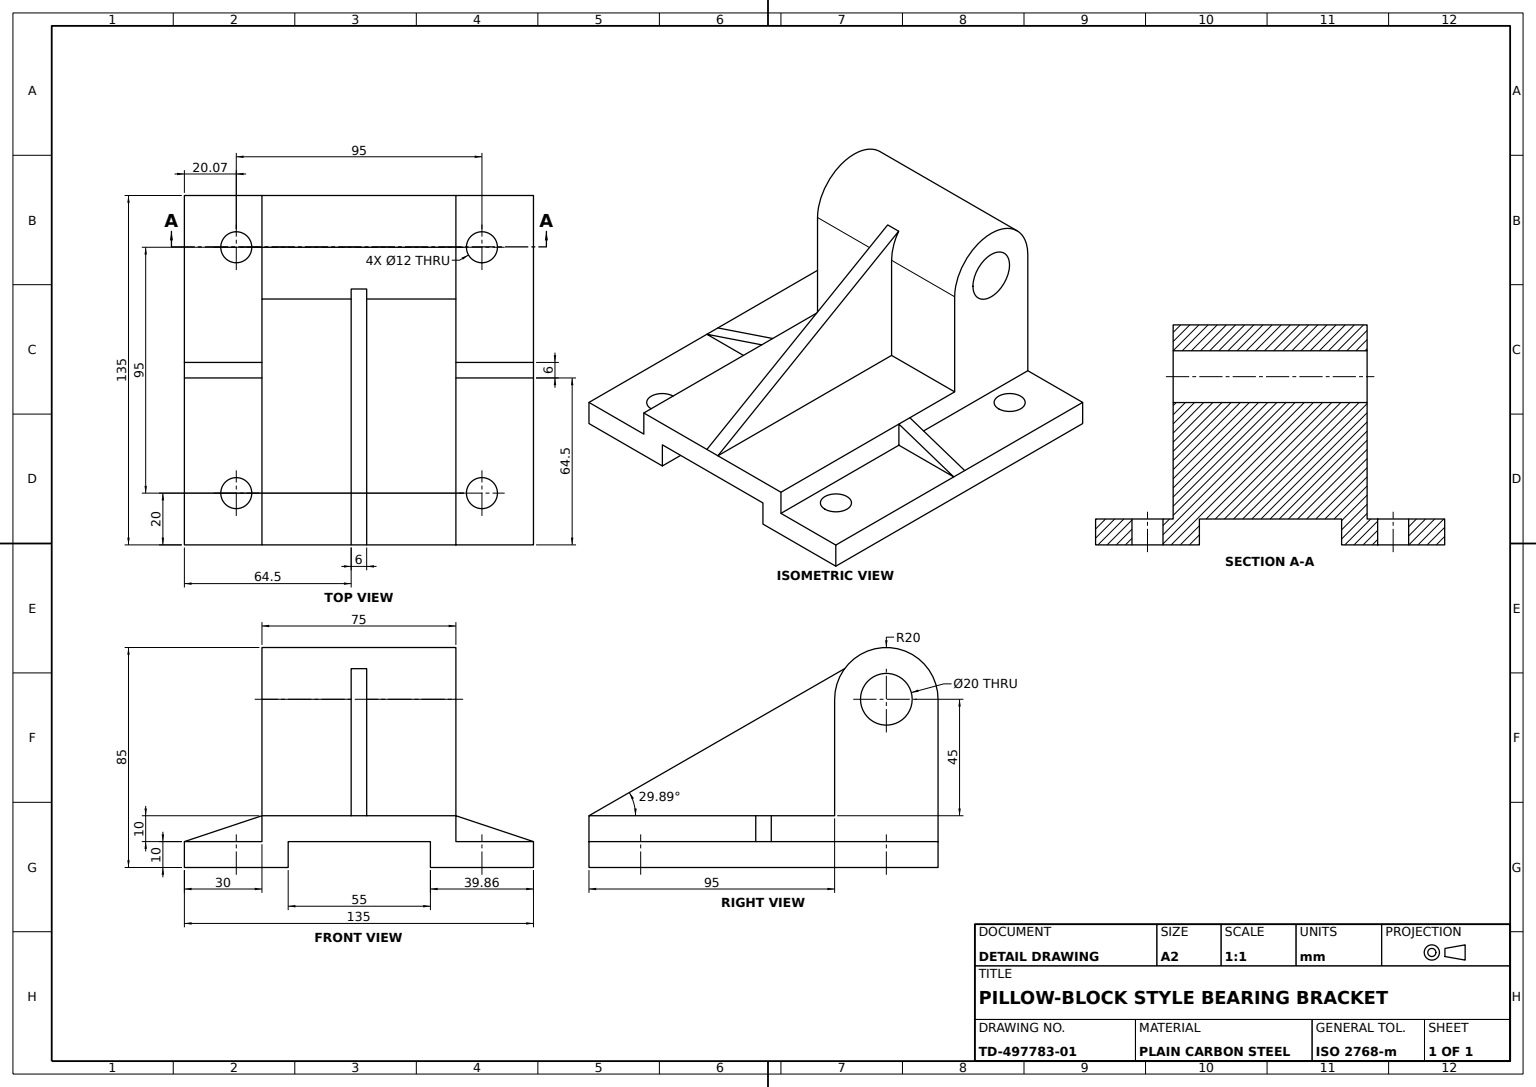
from build123d import *

# Parameters (mm, degrees)
BASE_PLATE_SKETCH_W     = 135
BASE_PLATE_SKETCH_H     = 20
BASE_PLATE_DEPTH        = 67.5
BOTTOM_CHANNEL_DEPTH    = 152.265495074
TOP_RECESS_SKETCH_W     = 30
TOP_RECESS_SKETCH_H     = 10
TOP_RECESS_DEPTH        = 152.265495074
UPRIGHT_LUG_SKETCH_R    = 10
UPRIGHT_LUG_DEPTH       = 75
SIDE_GUSSET_DEPTH       = 3
CENTRE_START            = -37.5
CENTRE_RIB_DEPTH        = 3
MOUNTING_HOLES_SKETCH_R = 6
MOUNTING_HOLES_12_DEPTH = 128.818230312


with BuildPart() as part:
    # Base Plate Sketch → Base Plate (new, symmetric)
    with BuildSketch(Plane.XY):
        Rectangle(BASE_PLATE_SKETCH_W, BASE_PLATE_SKETCH_H)
    extrude(amount=BASE_PLATE_DEPTH, both=True)

    # Bottom Channel Sketch → Bottom Channel (cut, through all)
    with BuildSketch(Plane.XY.offset(67.5)):
        Polygon((27.643184154, 0), (0, 0), (-27.356815846, 0), (-27.356815846, -10), (27.643184154, -10), align=None)
    extrude(amount=-BOTTOM_CHANNEL_DEPTH, mode=Mode.SUBTRACT)

    # Top Recess Sketch → Top Recess (cut, through all)
    with BuildSketch(Plane.XY.offset(67.5)):
        with Locations((-52.5, 5)):
            Rectangle(TOP_RECESS_SKETCH_W, TOP_RECESS_SKETCH_H)
        with Locations((52.5, 5)):
            Rectangle(TOP_RECESS_SKETCH_W, TOP_RECESS_SKETCH_H)
    extrude(amount=-TOP_RECESS_DEPTH, mode=Mode.SUBTRACT)

    # Upright Lug Sketch → Upright Lug (add)
    with BuildSketch(Plane(origin=(37.5, 0, 0), x_dir=(0, 0, -1), z_dir=(1, 0, 0))):
        with BuildLine():
            Line((67.5, 10), (67.5, 55))
            ThreePointArc((67.5, 55), (47.5, 75), (27.5, 55))
            Line((27.5, 55), (27.5, 10))
            Line((27.5, 10), (67.5, 10))
        make_face()
        with Locations((47.5, 55)):
            Circle(UPRIGHT_LUG_SKETCH_R, mode=Mode.SUBTRACT)
    extrude(amount=-UPRIGHT_LUG_DEPTH)

    # Side Gusset Sketch → Side Gusset (add, symmetric)
    with BuildSketch(Plane.XY):
        Polygon((-67.5, 0), (-37.5, 10), (-37.5, 0), align=None)
    side_gusset = extrude(amount=SIDE_GUSSET_DEPTH, both=True)

    # Side Gusset Mirror: Side Gusset across plane
    add(side_gusset.mirror(Plane(origin=(0, 0, 0), x_dir=(0, 0, 1), z_dir=(1, 0, 0))))

    # Centre Rib Sketch → Centre Rib (add, symmetric)
    with BuildSketch(Plane(origin=(37.5, 0, 0), x_dir=(0, 0, -1), z_dir=(1, 0, 0)).offset(CENTRE_START)):
        Polygon((-67.5, 10), (35.500032612, 69.198001073), (35.500032612, 10), (29.449687004, 10), align=None)
    extrude(amount=CENTRE_RIB_DEPTH, both=True)

    # Mounting Holes Sketch → Mounting Holes Ø12 (cut, through all)
    with BuildSketch(Plane.XZ.offset(10)):
        with Locations(Location((47.571592077, -47.5, 0), (0, 0, 270))):
            Circle(MOUNTING_HOLES_SKETCH_R)
        with Locations(Location((-47.428407923, -47.5, 0), (0, 0, 270))):
            Circle(MOUNTING_HOLES_SKETCH_R)
        with Locations(Location((-47.428407923, 47.5, 0), (0, 0, 270))):
            Circle(MOUNTING_HOLES_SKETCH_R)
        with Locations(Location((47.571592077, 47.5, 0), (0, 0, 270))):
            Circle(MOUNTING_HOLES_SKETCH_R)
    extrude(amount=-MOUNTING_HOLES_12_DEPTH, mode=Mode.SUBTRACT)


solid = part.part
